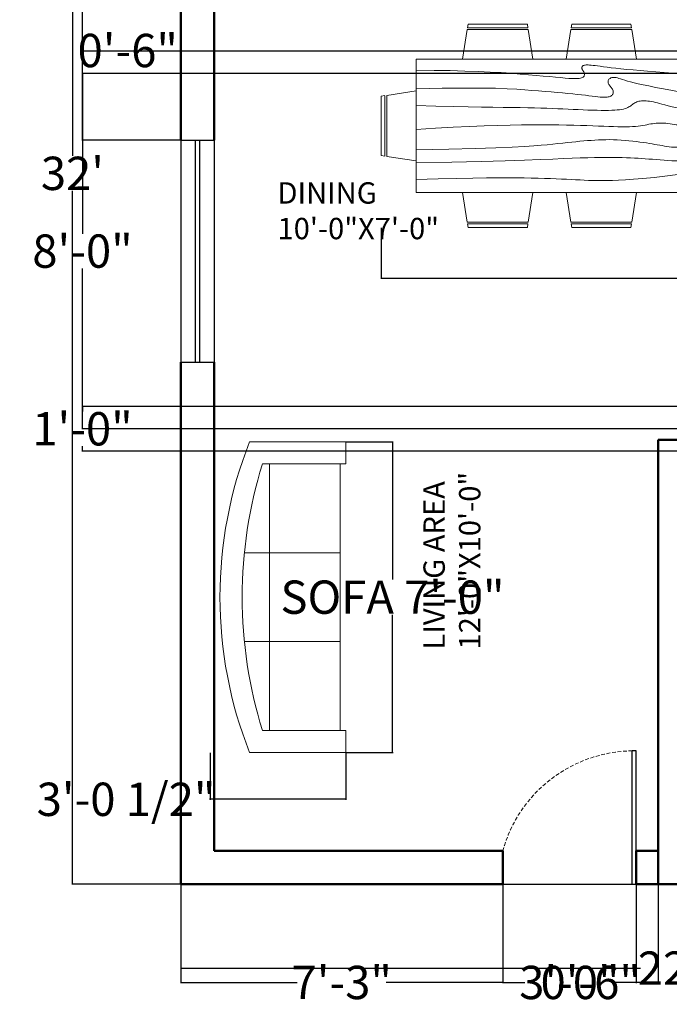
# Model space of a CAD drawing. Units: inches. Extents: x 4033 to 4435, y 499 to 1031.
# Tile 1 of 4: x 4042 to 4217, y 499 to 765. Entities that reach past the tile are written whole.
import ezdxf

# ---------------------------------------------------------------- set-up
doc = ezdxf.new("R2010")
doc.units = ezdxf.units.IN
doc.header["$MEASUREMENT"] = 0
doc.linetypes.add('DASHEDX2', pattern=[1.5, 1, -0.5])
for name, color, linetype, lineweight in [('A-ANNO-DIMS', 2, 'Continuous', 18), ('A-AREA-IDEN', 7, 'Continuous', 18), ('A-DOOR', 3, 'Continuous', 25), ('A-DOOR-SWNG', 3, 'DASHEDX2', 13), ('A-FURN', 8, 'Continuous', 18), ('A-WALL', 7, 'Continuous', 50)]:
    doc.layers.add(name, color=color, linetype=linetype, lineweight=lineweight)
doc.layers.add('A-GLAZ', color=177, linetype='Continuous', lineweight=25, true_color=0x293189)
doc.styles.get("Standard").update_dxf_attribs({"font": 'arial.ttf'})
doc.dimstyles.get("Standard").update_dxf_attribs({"dimtxt": 9, "dimasz": 0.18, "dimexe": 0.18, "dimexo": 0.0625, "dimgap": 0.09, "dimtad": 0, "dimtih": 1, "dimtoh": 1, "dimdec": 0, "dimzin": 0, "dimdsep": 46, "dimlunit": 3, "dimtxsty": 'Standard', "dimcen": 0.09, "dimadec": 0, "dimazin": 0, "dimtfac": 1, "dimtdec": 0, "dimtofl": 0, "dimtmove": 0, "dimatfit": 3, "dimfxl": 1, "dimtolj": 1, "dimtzin": 0, "dimarcsym": 0})

# ---------------------------------------------------------------- blocks, each defined once
blk = doc.blocks.new('Sofa - Roundback 7 ft.')
for p, q in [((-12.00002, -32.4421), (-12.00003, -6.5971)), ((11.99997, -32.4421), (11.99998, -6.5971)), ((-36.000027, -34), (-36.000027, -11.4696)), ((35.99998, -34), (35.99998, -11.4696)), ((-35.999844, -13.3819), (35.9998, -13.3819)), ((-36.000027, -32.4421), (35.99998, -32.4421))]:
    blk.add_line(p, q)
for points in [[(-36.000027, -34), (-42.000027, -34), (-42.000027, -8)], [(41.99998, -8), (41.99998, -34), (35.99998, -34)]]:
    blk.add_lwpolyline(points)
for centre, radius, start, end in [((0, -114.25), 114.25, 68.43141, 111.5686), ((-0.00001, -127.1968), 121.1968, 72.72033, 107.2797)]:
    blk.add_arc(centre, radius, start, end)
blk = doc.blocks.new('Dining Set - 36 x 72 in.')
for p, q in [((-22, 27.5), (-22.1562, 26.50042)), ((-22, 27.5), (-6, 27.5)), ((-5.8437, 26.49966), (-6, 27.5)), ((6, 27.5), (5.8438, 26.50042)), ((6, 27.5), (22, 27.5)), ((22.1563, 26.49966), (22, 27.5)), ((-22.2343, 26.00059), (-23.4847, 17.99762)), ((-22.2304, 26), (-5.7608, 26)), ((-5.8416, 26.5), (-22.1534, 26.5)), ((-4.5152, 17.99762), (-5.7655, 25.99926)), ((5.7657, 26.00059), (4.5153, 17.99762)), ((5.7696, 26), (22.2392, 26)), ((22.1584, 26.5), (5.8466, 26.5)), ((23.4848, 17.99762), (22.2345, 25.99926)), ((36, 18), (-36, 18)), ((-36, 18), (-36, -18)), ((36, -18), (36, 18)), ((-45.5, 8), (-44.5004, 8.15617)), ((-45.5, 8), (-45.5, -8)), ((-44.5, -8.15843), (-44.5, 8.15338)), ((-44.0006, 8.23428), (-35.9976, 9.48474)), ((-44, 8.23041), (-44, -8.23915)), ((44.0006, 8.23428), (35.9976, 9.48474)), ((44, 8.23041), (44, -8.23915)), ((44.5, -8.15843), (44.5, 8.15338)), ((45.5, 8), (44.5005, 8.15617)), ((45.5, 8), (45.5, -8)), ((-44.4997, -8.15631), (-45.5, -8)), ((-35.9976, -9.48476), (-43.9993, -8.2345)), ((35.9976, -9.48476), (43.9993, -8.2345)), ((44.4997, -8.15631), (45.5, -8)), ((-36, -18), (36, -18)), ((-22.2343, -26.0006), (-23.4847, -17.99762)), ((-4.5152, -17.99762), (-5.7655, -25.99928)), ((5.7657, -26.0006), (4.5153, -17.99762)), ((23.4848, -17.99762), (22.2345, -25.99928)), ((-22.2304, -26), (-5.7608, -26)), ((-22, -27.5), (-22.1562, -26.50044)), ((-5.8416, -26.5), (-22.1534, -26.5)), ((-5.8437, -26.49967), (-6, -27.5)), ((5.7696, -26), (22.2392, -26)), ((6, -27.5), (5.8438, -26.50044)), ((22.1584, -26.5), (5.8466, -26.5)), ((22.1563, -26.49967), (22, -27.5)), ((-22, -27.5), (-6, -27.5)), ((6, -27.5), (22, -27.5))]:
    blk.add_line(p, q)
for points in [[(-36, 15), (-31.1772, 14.97754), (-26.8079, 14.91406), (-22.8538, 14.81543), (-19.276, 14.6875), (-16.0362, 14.53613), (-13.0957, 14.36718), (-10.4159, 14.18652), (-7.9583, 14), (-5.6904, 13.81315), (-3.6035, 13.63021), (-1.6954, 13.45508), (0.0365, 13.29166), (1.5945, 13.14388), (2.9811, 13.01562), (4.1988, 12.9108), (5.25, 12.83333), (6.1393, 12.78613), (6.8802, 12.76823), (7.4883, 12.77767), (7.9792, 12.8125), (8.3685, 12.87077), (8.6719, 12.95052), (8.9049, 13.0498), (9.0833, 13.16666), (9.2205, 13.29899), (9.3216, 13.44401), (9.3895, 13.59879), (9.4271, 13.76041), (9.4373, 13.92594), (9.4232, 14.09245), (9.3875, 14.257), (9.3333, 14.41666), (9.2638, 14.56917), (9.1836, 14.71484), (9.0975, 14.85465), (9.0104, 14.98958), (8.9272, 15.1206), (8.8529, 15.2487), (8.7922, 15.37483), (8.75, 15.5), (8.7305, 15.62467), (8.7344, 15.74739), (8.7617, 15.86621), (8.8125, 15.97916), (8.8867, 16.08431), (8.9844, 16.17968), (9.1055, 16.26334), (9.25, 16.33333), (9.4189, 16.38802), (9.6172, 16.42708), (9.8506, 16.45052), (10.125, 16.45833), (10.4463, 16.45052), (10.8203, 16.42708), (11.2529, 16.38802), (11.75, 16.33333), (12.3184, 16.26318), (12.9694, 16.17838), (13.7151, 16.07991), (14.5677, 15.96875), (15.5395, 15.84586), (16.6426, 15.71224), (17.8893, 15.56884), (19.2917, 15.41666), (20.859, 15.25667), (22.5879, 15.08984), (24.4721, 14.91715), (26.5052, 14.73958), (28.6809, 14.5581), (30.9929, 14.3737), (33.4347, 14.18733), (36, 14)], [(-36, 10), (-28.9766, 10.14274), (-23.1725, 10.20442), (-18.4241, 10.19775), (-14.5677, 10.13541), (-11.4399, 10.03011), (-8.877, 9.89453), (-6.7154, 9.74137), (-4.7917, 9.58333), (-2.9698, 9.43082), (-1.2246, 9.28515), (0.4415, 9.14534), (2.026, 9.01041), (3.5266, 8.87939), (4.9408, 8.7513), (6.266, 8.62516), (7.5, 8.5), (8.6411, 8.37549), (9.6914, 8.2539), (10.6538, 8.13818), (11.5312, 8.03125), (12.3267, 7.93603), (13.043, 7.85547), (13.6831, 7.79248), (14.25, 7.75), (14.7471, 7.7303), (15.1797, 7.73307), (15.5537, 7.75732), (15.875, 7.80208), (16.1494, 7.86637), (16.3828, 7.94922), (16.5811, 8.04964), (16.75, 8.16666), (16.8944, 8.29915), (17.0143, 8.44531), (17.1089, 8.60319), (17.1771, 8.77083), (17.218, 8.94629), (17.2305, 9.1276), (17.2137, 9.31282), (17.1667, 9.5), (17.0895, 9.6875), (16.987, 9.875), (16.8649, 10.0625), (16.7292, 10.25), (16.5856, 10.4375), (16.4401, 10.625), (16.2985, 10.8125), (16.1667, 11), (16.05, 11.18733), (15.9518, 11.3737), (15.8752, 11.5581), (15.8229, 11.73958), (15.798, 11.91715), (15.8034, 12.08984), (15.842, 12.25667), (15.9167, 12.41666), (16.0295, 12.56836), (16.1784, 12.70833), (16.3605, 12.83268), (16.5729, 12.9375), (16.8127, 13.01888), (17.0768, 13.07291), (17.3625, 13.0957), (17.6667, 13.08333), (17.9894, 13.03312), (18.3418, 12.94726), (18.7382, 12.82918), (19.1927, 12.68229), (19.7195, 12.51001), (20.3327, 12.31575), (21.0465, 12.10294), (21.875, 11.875), (22.8357, 11.63354), (23.959, 11.37304), (25.2786, 11.08618), (26.8282, 10.76562), (28.6414, 10.40405), (30.752, 9.99414), (33.1936, 9.52856), (36, 9)], [(-36, 5.5), (-30.7157, 5.3348), (-26.069, 5.20963), (-21.9946, 5.11767), (-18.4271, 5.05208), (-15.3009, 5.00602), (-12.5508, 4.97265), (-10.1112, 4.94515), (-7.9167, 4.91666), (-5.909, 4.88167), (-4.0586, 4.83984), (-2.3429, 4.79215), (-0.7396, 4.73958), (0.7739, 4.6831), (2.22, 4.6237), (3.6213, 4.56233), (5, 4.5), (6.373, 4.43782), (7.7344, 4.3776), (9.0723, 4.32129), (10.375, 4.27083), (11.6309, 4.22819), (12.8281, 4.19531), (13.9551, 4.17415), (15, 4.16666), (15.954, 4.17448), (16.819, 4.19791), (17.6001, 4.23698), (18.3021, 4.29166), (18.9299, 4.36198), (19.4883, 4.44791), (19.9823, 4.54948), (20.4167, 4.66666), (20.7969, 4.79899), (21.1302, 4.94401), (21.4245, 5.09879), (21.6875, 5.26041), (21.9271, 5.42594), (22.1511, 5.59245), (22.3672, 5.757), (22.5834, 5.91666), (22.8065, 6.06868), (23.0404, 6.21093), (23.2879, 6.34147), (23.5521, 6.45833), (23.8358, 6.55957), (24.142, 6.64323), (24.4735, 6.70735), (24.8334, 6.75), (25.2235, 6.76969), (25.642, 6.76692), (26.0858, 6.74267), (26.5521, 6.69791), (27.0379, 6.63362), (27.5404, 6.55078), (28.0565, 6.45036), (28.5834, 6.33333), (29.1242, 6.19987), (29.7071, 6.04687), (30.3661, 5.87044), (31.1354, 5.66666), (32.0493, 5.43164), (33.142, 5.16146), (34.4475, 4.85221), (36, 4.5)], [(-36, -1), (-30.7915, -0.6591), (-26.0195, -0.38216), (-21.6519, -0.16284), (-17.6563, 0.00521), (-14.0005, 0.12833), (-10.6523, 0.21289), (-7.5796, 0.26522), (-4.75, 0.29166), (-2.134, 0.29793), (0.2878, 0.28711), (2.5317, 0.26163), (4.6146, 0.22396), (6.5529, 0.17651), (8.3633, 0.12174), (10.0623, 0.06209), (11.6667, 0), (13.1899, -0.06201), (14.6341, -0.1211), (15.9982, -0.17432), (17.2813, -0.21875), (18.4823, -0.25147), (19.6003, -0.26953), (20.6343, -0.27002), (21.5834, -0.25), (22.4481, -0.20768), (23.2357, -0.14584), (23.9549, -0.06836), (24.6146, 0.02083), (25.2235, 0.11784), (25.7904, 0.21875), (26.3241, 0.31966), (26.8334, 0.41666), (27.3265, 0.50618), (27.8099, 0.58593), (28.2894, 0.65397), (28.7709, 0.70833), (29.2601, 0.74707), (29.763, 0.76823), (30.2855, 0.76985), (30.8334, 0.75), (31.4088, 0.70784), (31.9994, 0.64713), (32.589, 0.57275), (33.1615, 0.48958), (33.7008, 0.4025), (34.1908, 0.3164), (34.6153, 0.23616), (34.9584, 0.16666), (35.2099, 0.11165), (35.3848, 0.07031), (35.504, 0.04069), (35.5886, 0.02083), (35.6594, 0.00879), (35.7377, 0.0026), (35.8442, 0.00032), (36, 0)], [(-36, -6.5), (-27.1843, -6.31267), (-20.084, -6.1263), (-14.469, -5.9419), (-10.1094, -5.76042), (-6.7752, -5.58285), (-4.2363, -5.41016), (-2.2629, -5.24333), (-0.625, -5.08334), (0.8708, -4.93099), (2.2715, -4.78646), (3.5872, -4.64974), (4.8281, -4.52084), (6.0046, -4.39974), (7.127, -4.28646), (8.2053, -4.18099), (9.25, -4.08334), (10.2705, -3.99382), (11.2734, -3.91407), (12.2647, -3.84603), (13.25, -3.79167), (14.2354, -3.75293), (15.2266, -3.73177), (16.2295, -3.73015), (17.25, -3.75), (18.2912, -3.79248), (19.3451, -3.85547), (20.4009, -3.93604), (21.4479, -4.03125), (22.4754, -4.13819), (23.4727, -4.25391), (24.4289, -4.37549), (25.3334, -4.5), (26.1785, -4.62492), (26.9694, -4.74935), (27.7145, -4.87281), (28.4219, -4.99479), (29.1, -5.11483), (29.7572, -5.23242), (30.4016, -5.34709), (31.0417, -5.45834), (31.6837, -5.56437), (32.3262, -5.65821), (32.9658, -5.73153), (33.599, -5.77604), (34.2224, -5.78345), (34.8327, -5.74545), (35.4264, -5.65373), (36, -5.5)], [(-36, -10), (-26.4022, -9.81299), (-18.4675, -9.62891), (-11.9839, -9.45069), (-6.7396, -9.28125), (-2.5226, -9.12354), (0.8789, -8.98047), (3.6769, -8.85498), (6.0833, -8.75), (8.2767, -8.66765), (10.3021, -8.60677), (12.1712, -8.56543), (13.8958, -8.54167), (15.4876, -8.53353), (16.9583, -8.53907), (18.3197, -8.55632), (19.5834, -8.58334), (20.7616, -8.61841), (21.8685, -8.66081), (22.9188, -8.71004), (23.9271, -8.76563), (24.9081, -8.82707), (25.8763, -8.89388), (26.8465, -8.96558), (27.8334, -9.04167), (28.8474, -9.12118), (29.8828, -9.20117), (30.93, -9.27824), (31.9792, -9.34896), (33.0205, -9.40991), (34.0443, -9.45768), (35.0407, -9.48885), (36, -9.5)], [(-36, -14.5), (-30.0881, -14.33513), (-25.0332, -14.21224), (-20.7312, -14.12647), (-17.0781, -14.07292), (-13.97, -14.04671), (-11.3027, -14.04297), (-8.9724, -14.05681), (-6.875, -14.08334), (-4.9224, -14.11833), (-3.0905, -14.16016), (-1.3709, -14.20785), (0.2448, -14.26042), (1.7647, -14.3169), (3.1973, -14.3763), (4.5507, -14.43767), (5.8333, -14.5), (7.0554, -14.5621), (8.235, -14.62175), (9.3922, -14.67652), (10.5469, -14.72396), (11.7192, -14.76164), (12.929, -14.78711), (14.1965, -14.79794), (15.5417, -14.79167), (16.9933, -14.76424), (18.6152, -14.70508), (20.4804, -14.60197), (22.6615, -14.44271), (25.2312, -14.21509), (28.2624, -13.9069), (31.8277, -13.50594), (36, -13)]]:
    blk.add_lwpolyline(points)
blk = doc.blocks.new('*D9')
at = {"layer": 'A-ANNO-DIMS', "color": 0, "lineweight": -2, "transparency": 16777216}
for p, q in [((4085.18, 531.19), (4085.18, 508.39)), ((4349.18, 531.19), (4349.18, 508.39)), ((4085.36, 508.57), (4209.37, 508.57)), ((4349, 508.57), (4224.98, 508.57))]:
    blk.add_line(p, q, dxfattribs=at)
at = {"layer": 'A-ANNO-DIMS', "color": 0, "transparency": 16777216}
for points in [[(4085.36, 508.6), (4085.36, 508.54), (4085.18, 508.57)], [(4349, 508.6), (4349, 508.54), (4349.18, 508.57)]]:
    blk.add_solid(points, dxfattribs=at)
at = {"layer": 'Defpoints', "color": 0, "transparency": 16777216}
for p in [(4085.18, 531.25), (4349.18, 531.25), (4349.18, 508.57)]:
    blk.add_point(p, dxfattribs=at)
at = {"layer": 'A-ANNO-DIMS', "color": 0, "transparency": 16777216, "insert": (4217.18, 508.57), "char_height": 9, "attachment_point": 5}
blk.add_mtext("\\A1;22'", dxfattribs=at)
blk = doc.blocks.new('*D10')
at = {"layer": 'A-ANNO-DIMS', "color": 0, "lineweight": -2, "transparency": 16777216}
for p, q in [((4085.12, 915.25), (4055.73, 915.25)), ((4055.91, 915.07), (4055.91, 727.94)), ((4055.91, 531.43), (4055.91, 718.56)), ((4085.12, 531.25), (4055.73, 531.25))]:
    blk.add_line(p, q, dxfattribs=at)
at = {"layer": 'A-ANNO-DIMS', "color": 0, "transparency": 16777216}
for points in [[(4055.88, 915.07), (4055.94, 915.07), (4055.91, 915.25)], [(4055.88, 531.43), (4055.94, 531.43), (4055.91, 531.25)]]:
    blk.add_solid(points, dxfattribs=at)
at = {"layer": 'Defpoints', "color": 0, "transparency": 16777216}
for p in [(4055.91, 915.25), (4085.18, 915.25), (4085.18, 531.25)]:
    blk.add_point(p, dxfattribs=at)
at = {"layer": 'A-ANNO-DIMS', "color": 0, "transparency": 16777216, "insert": (4055.91, 723.25), "char_height": 9, "attachment_point": 5}
blk.add_mtext("\\A1;32'", dxfattribs=at)
blk = doc.blocks.new('WIN-60IN')
for p, q in [((0, 0), (0, 9)), ((0, 9), (60, 9)), ((60, 0), (60, 9)), ((0, 5.1), (60, 5.1)), ((0, 3.9), (60, 3.9)), ((0, 0), (60, 0))]:
    blk.add_line(p, q)
blk = doc.blocks.new('*D22')
at = {"layer": 'A-ANNO-DIMS', "color": 0, "lineweight": -2, "transparency": 16777216}
for p, q in [((4129.84, 650.77), (4142.56, 650.77)), ((4142.38, 650.59), (4142.38, 613.52)), ((4142.38, 566.95), (4142.38, 604.02)), ((4129.84, 566.77), (4142.56, 566.77))]:
    blk.add_line(p, q, dxfattribs=at)
at = {"layer": 'A-ANNO-DIMS', "color": 0, "transparency": 16777216}
for points in [[(4142.35, 650.59), (4142.41, 650.59), (4142.38, 650.77)], [(4142.35, 566.95), (4142.41, 566.95), (4142.38, 566.77)]]:
    blk.add_solid(points, dxfattribs=at)
at = {"layer": 'Defpoints', "color": 0, "transparency": 16777216}
for p in [(4129.78, 650.77), (4129.78, 566.77), (4142.38, 566.77)]:
    blk.add_point(p, dxfattribs=at)
at = {"layer": 'A-ANNO-DIMS', "color": 0, "transparency": 16777216, "insert": (4142.38, 608.77), "char_height": 9, "attachment_point": 5}
blk.add_mtext('\\A1;SOFA 7\'-0"', dxfattribs=at)
blk = doc.blocks.new('*D23')
at = {"layer": 'A-ANNO-DIMS', "color": 0, "lineweight": -2, "transparency": 16777216}
for p, q in [((4093.11, 566.71), (4093.11, 553.99)), ((4129.78, 566.71), (4129.78, 553.99)), ((4093.11, 554.17), (4092.93, 554.17)), ((4129.6, 554.17), (4093.29, 554.17))]:
    blk.add_line(p, q, dxfattribs=at)
at = {"layer": 'A-ANNO-DIMS', "color": 0, "transparency": 16777216}
for points in [[(4093.29, 554.2), (4093.29, 554.14), (4093.11, 554.17)], [(4129.6, 554.2), (4129.6, 554.14), (4129.78, 554.17)]]:
    blk.add_solid(points, dxfattribs=at)
at = {"layer": 'Defpoints', "color": 0, "transparency": 16777216}
for p in [(4093.11, 566.77), (4129.78, 566.77), (4093.11, 554.17)]:
    blk.add_point(p, dxfattribs=at)
at = {"layer": 'A-ANNO-DIMS', "color": 0, "transparency": 16777216, "insert": (4070.4, 554.17), "char_height": 9, "attachment_point": 5}
blk.add_mtext('\\A1;3\'-0 1/2"', dxfattribs=at)
blk = doc.blocks.new('*D30')
at = {"layer": 'A-ANNO-DIMS', "color": 0, "lineweight": -2, "transparency": 16777216}
for p, q in [((4139.32, 708.52), (4139.32, 694.75)), ((4230.32, 708.52), (4230.32, 694.75)), ((4139.5, 694.93), (4230.14, 694.93)), ((4230.32, 694.93), (4230.5, 694.93))]:
    blk.add_line(p, q, dxfattribs=at)
at = {"layer": 'A-ANNO-DIMS', "color": 0, "transparency": 16777216}
for points in [[(4139.5, 694.96), (4139.5, 694.9), (4139.32, 694.93)], [(4230.14, 694.96), (4230.14, 694.9), (4230.32, 694.93)]]:
    blk.add_solid(points, dxfattribs=at)
at = {"layer": 'Defpoints', "color": 0, "transparency": 16777216}
for p in [(4139.32, 708.58), (4230.32, 708.58), (4230.32, 694.93)]:
    blk.add_point(p, dxfattribs=at)
at = {"layer": 'A-ANNO-DIMS', "color": 0, "transparency": 16777216, "insert": (4280.05, 694.93), "char_height": 9, "attachment_point": 5}
blk.add_mtext('\\A1;DINING SET 7\'-7"', dxfattribs=at)
blk = doc.blocks.new('*D38')
at = {"layer": 'A-ANNO-DIMS', "color": 0, "lineweight": -2, "transparency": 16777216}
for p, q in [((4085.12, 915.25), (4058.45, 915.25)), ((4058.63, 915.07), (4058.63, 828.44)), ((4058.63, 732.43), (4058.63, 819.06)), ((4085.12, 732.25), (4058.45, 732.25))]:
    blk.add_line(p, q, dxfattribs=at)
at = {"layer": 'A-ANNO-DIMS', "color": 0, "transparency": 16777216}
for points in [[(4058.6, 915.07), (4058.66, 915.07), (4058.63, 915.25)], [(4058.6, 732.43), (4058.66, 732.43), (4058.63, 732.25)]]:
    blk.add_solid(points, dxfattribs=at)
at = {"layer": 'Defpoints', "color": 0, "transparency": 16777216}
for p in [(4058.63, 915.25), (4085.18, 915.25), (4085.18, 732.25)]:
    blk.add_point(p, dxfattribs=at)
at = {"layer": 'A-ANNO-DIMS', "color": 0, "transparency": 16777216, "insert": (4058.63, 823.75), "char_height": 9, "attachment_point": 5}
blk.add_mtext('\\A1;15\'-3"', dxfattribs=at)
blk = doc.blocks.new('*D39')
at = {"layer": 'A-ANNO-DIMS', "color": 0, "lineweight": -2, "transparency": 16777216}
for p, q in [((4085.18, 531.19), (4085.18, 504.52)), ((4172.18, 531.19), (4172.18, 504.52)), ((4085.36, 504.7), (4116.66, 504.7)), ((4172, 504.7), (4140.69, 504.7))]:
    blk.add_line(p, q, dxfattribs=at)
at = {"layer": 'A-ANNO-DIMS', "color": 0, "transparency": 16777216}
for points in [[(4085.36, 504.73), (4085.36, 504.67), (4085.18, 504.7)], [(4172, 504.73), (4172, 504.67), (4172.18, 504.7)]]:
    blk.add_solid(points, dxfattribs=at)
at = {"layer": 'Defpoints', "color": 0, "transparency": 16777216}
for p in [(4085.18, 531.25), (4172.18, 531.25), (4085.18, 504.7)]:
    blk.add_point(p, dxfattribs=at)
at = {"layer": 'A-ANNO-DIMS', "color": 0, "transparency": 16777216, "insert": (4128.68, 504.7), "char_height": 9, "attachment_point": 5}
blk.add_mtext('\\A1;7\'-3"', dxfattribs=at)
blk = doc.blocks.new('*D40')
at = {"layer": 'A-ANNO-DIMS', "color": 0, "lineweight": -2, "transparency": 16777216}
for p, q in [((4172.18, 531.19), (4172.18, 504.52)), ((4208.18, 531.19), (4208.18, 504.52)), ((4172.36, 504.7), (4178.13, 504.7)), ((4208, 504.7), (4202.23, 504.7))]:
    blk.add_line(p, q, dxfattribs=at)
at = {"layer": 'A-ANNO-DIMS', "color": 0, "transparency": 16777216}
for points in [[(4172.36, 504.73), (4172.36, 504.67), (4172.18, 504.7)], [(4208, 504.73), (4208, 504.67), (4208.18, 504.7)]]:
    blk.add_solid(points, dxfattribs=at)
at = {"layer": 'Defpoints', "color": 0, "transparency": 16777216}
for p in [(4172.18, 531.25), (4208.18, 531.25), (4172.18, 504.7)]:
    blk.add_point(p, dxfattribs=at)
at = {"layer": 'A-ANNO-DIMS', "color": 0, "transparency": 16777216, "insert": (4190.18, 504.7), "char_height": 9, "attachment_point": 5}
blk.add_mtext('\\A1;3\'-0"', dxfattribs=at)
blk = doc.blocks.new('*D41')
at = {"layer": 'A-ANNO-DIMS', "color": 0, "lineweight": -2, "transparency": 16777216}
for p, q in [((4208.18, 531.19), (4208.18, 504.52)), ((4214.18, 531.19), (4214.18, 504.52)), ((4208.18, 504.7), (4208, 504.7)), ((4214, 504.7), (4208.36, 504.7))]:
    blk.add_line(p, q, dxfattribs=at)
at = {"layer": 'A-ANNO-DIMS', "color": 0, "transparency": 16777216}
for points in [[(4208.36, 504.73), (4208.36, 504.67), (4208.18, 504.7)], [(4214, 504.73), (4214, 504.67), (4214.18, 504.7)]]:
    blk.add_solid(points, dxfattribs=at)
at = {"layer": 'Defpoints', "color": 0, "transparency": 16777216}
for p in [(4208.18, 531.25), (4214.18, 531.25), (4208.18, 504.7)]:
    blk.add_point(p, dxfattribs=at)
at = {"layer": 'A-ANNO-DIMS', "color": 0, "transparency": 16777216, "insert": (4195.95, 504.7), "char_height": 9, "attachment_point": 5}
blk.add_mtext('\\A1;0\'-6"', dxfattribs=at)
blk = doc.blocks.new('*D54')
at = {"layer": 'A-ANNO-DIMS', "color": 0, "lineweight": -2, "transparency": 16777216}
for p, q in [((4280.12, 750.25), (4058.45, 750.25)), ((4058.63, 750.07), (4058.63, 706.94)), ((4058.63, 654.43), (4058.63, 697.56)), ((4280.12, 654.25), (4058.45, 654.25))]:
    blk.add_line(p, q, dxfattribs=at)
at = {"layer": 'A-ANNO-DIMS', "color": 0, "transparency": 16777216}
for points in [[(4058.6, 750.07), (4058.66, 750.07), (4058.63, 750.25)], [(4058.6, 654.43), (4058.66, 654.43), (4058.63, 654.25)]]:
    blk.add_solid(points, dxfattribs=at)
at = {"layer": 'Defpoints', "color": 0, "transparency": 16777216}
for p in [(4058.63, 750.25), (4280.18, 750.25), (4280.18, 654.25)]:
    blk.add_point(p, dxfattribs=at)
at = {"layer": 'A-ANNO-DIMS', "color": 0, "transparency": 16777216, "insert": (4058.63, 702.25), "char_height": 9, "attachment_point": 5}
blk.add_mtext('\\A1;8\'-0"', dxfattribs=at)
blk = doc.blocks.new('*D55')
at = {"layer": 'A-ANNO-DIMS', "color": 0, "lineweight": -2, "transparency": 16777216}
for p, q in [((4280.12, 756.25), (4058.45, 756.25)), ((4058.63, 756.25), (4058.63, 756.43)), ((4058.63, 756.43), (4058.81, 756.43)), ((4058.63, 750.43), (4058.63, 756.07)), ((4280.12, 750.25), (4058.45, 750.25))]:
    blk.add_line(p, q, dxfattribs=at)
at = {"layer": 'A-ANNO-DIMS', "color": 0, "transparency": 16777216}
for points in [[(4058.6, 756.07), (4058.66, 756.07), (4058.63, 756.25)], [(4058.6, 750.43), (4058.66, 750.43), (4058.63, 750.25)]]:
    blk.add_solid(points, dxfattribs=at)
at = {"layer": 'Defpoints', "color": 0, "transparency": 16777216}
for p in [(4058.63, 756.25), (4280.18, 756.25), (4280.18, 750.25)]:
    blk.add_point(p, dxfattribs=at)
at = {"layer": 'A-ANNO-DIMS', "color": 0, "transparency": 16777216, "insert": (4070.86, 756.43), "char_height": 9, "attachment_point": 5}
blk.add_mtext('\\A1;0\'-6"', dxfattribs=at)
blk = doc.blocks.new('*D58')
at = {"layer": 'A-ANNO-DIMS', "color": 0, "lineweight": -2, "transparency": 16777216}
for p, q in [((4274.12, 660.25), (4058.45, 660.25)), ((4058.63, 660.07), (4058.63, 658.94)), ((4058.63, 648.43), (4058.63, 649.56)), ((4274.12, 648.25), (4058.45, 648.25))]:
    blk.add_line(p, q, dxfattribs=at)
at = {"layer": 'A-ANNO-DIMS', "color": 0, "transparency": 16777216}
for points in [[(4058.6, 660.07), (4058.66, 660.07), (4058.63, 660.25)], [(4058.6, 648.43), (4058.66, 648.43), (4058.63, 648.25)]]:
    blk.add_solid(points, dxfattribs=at)
at = {"layer": 'Defpoints', "color": 0, "transparency": 16777216}
for p in [(4058.63, 660.25), (4274.18, 660.25), (4274.18, 648.25)]:
    blk.add_point(p, dxfattribs=at)
at = {"layer": 'A-ANNO-DIMS', "color": 0, "transparency": 16777216, "insert": (4058.63, 654.25), "char_height": 9, "attachment_point": 5}
blk.add_mtext('\\A1;1\'-0"', dxfattribs=at)

msp = doc.modelspace()

# ---------------------------------------------------------------- linework, layer by layer
at = {"layer": 'A-DOOR'}
for p, q in [((4207.18, 531.25), (4207.18, 567.25)), ((4208.18, 567.25), (4207.18, 567.25)), ((4208.18, 531.25), (4208.18, 567.25)), ((4172.18, 531.25), (4208.18, 531.25))]:
    msp.add_line(p, q, dxfattribs=at)
at = {"layer": 'A-DOOR-SWNG'}
msp.add_arc((4207.68, 530.42), 36.84, 90.7777, 164.5175, dxfattribs=at)
at = {"layer": 'A-WALL'}
for p, q in [((4094.18, 780.25), (4094.18, 732.25)), ((4085.18, 768.25), (4085.18, 732.25)), ((4085.18, 672.25), (4085.18, 531.25)), ((4094.18, 672.25), (4094.18, 540.25)), ((4214.18, 651.25), (4214.18, 531.25)), ((4226.18, 651.25), (4214.18, 651.25)), ((4094.18, 540.25), (4172.18, 540.25)), ((4172.18, 540.25), (4172.18, 531.25)), ((4208.18, 540.25), (4208.18, 531.25)), ((4208.18, 540.25), (4214.18, 540.25)), ((4085.18, 531.25), (4172.18, 531.25)), ((4208.18, 531.25), (4220.18, 531.25))]:
    msp.add_line(p, q, dxfattribs=at)

# ---------------------------------------------------------------- block references
at = {"layer": 'A-FURN'}
msp.add_blockref('Dining Set - 36 x 72 in.', (4184.82, 736.08), dxfattribs=at)
at = {"layer": 'A-FURN', "xscale": -1, "rotation": 90}
msp.add_blockref('Sofa - Roundback 7 ft.', (4095.78, 608.77), dxfattribs=at)
at = {"layer": 'A-GLAZ', "rotation": 270.0000000000011}
msp.add_blockref('WIN-60IN', (4085.18, 732.25), dxfattribs=at)

# ---------------------------------------------------------------- texts
at = {"layer": 'A-AREA-IDEN', "insert": (4111.32, 720.84), "char_height": 5.7683, "attachment_point": 1}
msp.add_mtext_dynamic_manual_height_columns('DINING\\P10\'-0"X7\'-0"', width=2.1401, gutter_width=28.84, heights=[0], dxfattribs=at)
at = {"layer": 'A-AREA-IDEN', "insert": (4150.75, 594.62), "char_height": 5.7683, "attachment_point": 1, "rotation": 90}
msp.add_mtext_dynamic_manual_height_columns('LIVING AREA\\P12\'-0"X10\'-0"', width=58.4768, gutter_width=28.84, heights=[0], dxfattribs=at)

# ---------------------------------------------------------------- dimensions: what is measured, and where the dimension line sits
at = {"layer": 'A-ANNO-DIMS'}
for base, p1, p2, angle, override, picture, middle in [((4058.63, 915.25), (4085.18, 732.25), (4085.18, 915.25), 90, {"dimdec": 1, "dimlfac": 1, "dimrnd": 0, "dimzin": 1, "dimdsep": 46, "dimlunit": 4, "dimfrac": 2}, '*D38', (4058.63, 823.75)), ((4055.91, 915.25), (4085.18, 531.25), (4085.18, 915.25), 90, {"dimclrd": 0, "dimclre": 0, "dimclrt": 0}, '*D10', (4055.91, 723.25)), ((4058.63, 756.25), (4280.18, 750.25), (4280.18, 756.25), 90, {"dimdec": 1, "dimlfac": 1, "dimrnd": 0, "dimzin": 1, "dimdsep": 46, "dimlunit": 4, "dimfrac": 2}, '*D55', (4070.86, 756.43)), ((4058.63, 750.25), (4280.18, 654.25), (4280.18, 750.25), 90, {"dimdec": 1, "dimlfac": 1, "dimrnd": 0, "dimzin": 1, "dimdsep": 46, "dimlunit": 4, "dimfrac": 2}, '*D54', (4058.63, 702.25)), ((4058.63, 660.25), (4274.18, 648.25), (4274.18, 660.25), 90, {"dimdec": 1, "dimlfac": 1, "dimrnd": 0, "dimzin": 1, "dimdsep": 46, "dimlunit": 4, "dimfrac": 2}, '*D58', (4058.63, 654.25)), ((4093.11, 554.17), (4129.78, 566.77), (4093.11, 566.77), 180, {"dimdec": 1, "dimlfac": 1, "dimrnd": 0, "dimzin": 1, "dimdsep": 46, "dimlunit": 4, "dimfrac": 2}, '*D23', (4070.4, 554.17)), ((4085.18, 504.7), (4172.18, 531.25), (4085.18, 531.25), 180, {"dimdec": 1, "dimlfac": 1, "dimrnd": 0, "dimzin": 1, "dimdsep": 46, "dimlunit": 4, "dimfrac": 2}, '*D39', (4128.68, 504.7)), ((4172.18, 504.7), (4208.18, 531.25), (4172.18, 531.25), 180, {"dimdec": 1, "dimlfac": 1, "dimrnd": 0, "dimzin": 1, "dimdsep": 46, "dimlunit": 4, "dimfrac": 2}, '*D40', (4190.18, 504.7)), ((4208.18, 504.7), (4214.18, 531.25), (4208.18, 531.25), 180, {"dimdec": 1, "dimlfac": 1, "dimrnd": 0, "dimzin": 1, "dimdsep": 46, "dimlunit": 4, "dimfrac": 2}, '*D41', (4195.95, 504.7))]:
    dim = msp.add_linear_dim(base=base, p1=p1, p2=p2, angle=angle, dimstyle='Standard', override=override, dxfattribs=at)
    dim.commit()
    dim.dimension.update_dxf_attribs({"geometry": picture, "text_midpoint": middle})
dim = msp.add_linear_dim(base=(4230.32, 694.93), p1=(4139.32, 708.58), p2=(4230.32, 708.58), text='DINING SET <>', dimstyle='Standard', override={"dimdec": 1, "dimlfac": 1, "dimrnd": 0, "dimzin": 1, "dimdsep": 46, "dimlunit": 4, "dimfrac": 2}, dxfattribs=at)
dim.commit()
dim.dimension.update_dxf_attribs({"geometry": '*D30', "text_midpoint": (4280.05, 694.93)})
dim = msp.add_linear_dim(base=(4142.38, 566.77), p1=(4129.78, 650.77), p2=(4129.78, 566.77), angle=270, text='SOFA <>', dimstyle='Standard', override={"dimdec": 1, "dimlfac": 1, "dimrnd": 0, "dimzin": 1, "dimdsep": 46, "dimlunit": 4, "dimfrac": 2}, dxfattribs=at)
dim.commit()
dim.dimension.update_dxf_attribs({"geometry": '*D22', "text_midpoint": (4142.38, 608.77)})
dim = msp.add_linear_dim(base=(4349.18, 508.57), p1=(4085.18, 531.25), p2=(4349.18, 531.25), dimstyle='Standard', override={"dimclrd": 0, "dimclre": 0, "dimclrt": 0}, dxfattribs=at)
dim.commit()
dim.dimension.update_dxf_attribs({"geometry": '*D9', "text_midpoint": (4217.18, 508.57)})

doc.saveas('drawing.dxf')
